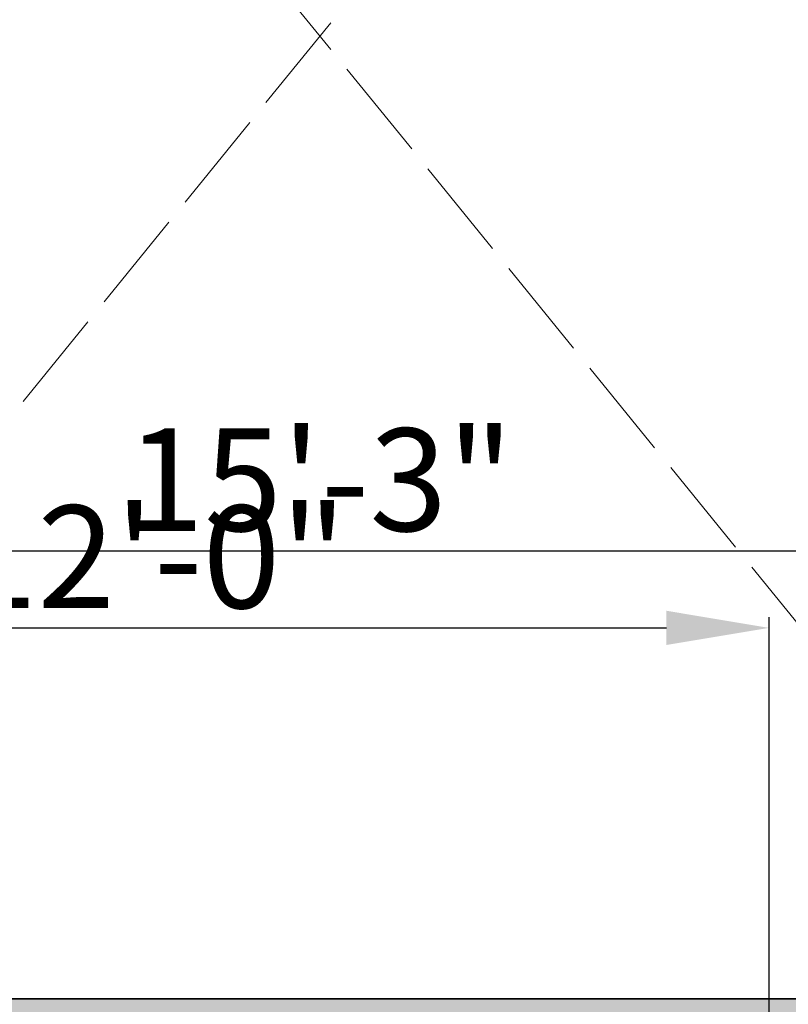
# Model space of a CAD drawing. Units: inches. Extents: x 2083 to 3317, y 1141 to 2115.
# Tile 82 of 256: x 2292 to 2382, y 1477 to 1592. Entities that reach past the tile are written whole.
import ezdxf

# ---------------------------------------------------------------- set-up
doc = ezdxf.new("R2010")
doc.units = ezdxf.units.IN
doc.linetypes.add('ACAD_ISO02W100', pattern=[15, 12, -3])
for name, color, linetype, lineweight in [('A-ANNO-DIMS', 2, 'Continuous', 18), ('A-FLOR-OPEN', 8, 'ACAD_ISO02W100', 13), ('A-WALL', 7, 'Continuous', 35)]:
    doc.layers.add(name, color=color, linetype=linetype, lineweight=lineweight)
doc.layers.add('A-WALL-PATT', color=251, linetype='Continuous', lineweight=13, true_color=0x636466)
doc.styles.get("Standard").update_dxf_attribs({"font": 'arial.ttf'})
doc.dimstyles.new('ISO-25', dxfattribs={"dimtxt": 12, "dimasz": 12, "dimexe": 1.25, "dimexo": 0.625, "dimtad": 1, "dimlunit": 3, "dimtxsty": 'Standard', "dimcen": 2.5, "dimadec": 0, "dimazin": 0, "dimtfac": 1, "dimtmove": 0, "dimatfit": 3, "dimfxl": 1, "dimarcsym": 0})

# ---------------------------------------------------------------- blocks, each defined once
blk = doc.blocks.new('*D30')
at = {"layer": 'A-ANNO-DIMS', "color": 0, "lineweight": -2, "transparency": 16777216}
for p, q in [((2240.02, 1445.27), (2240.02, 1448.05)), ((2254.33, 1445.27), (2254.33, 1448.05)), ((2228.02, 1446.8), (2216.02, 1446.8)), ((2240.02, 1446.8), (2254.33, 1446.8)), ((2266.33, 1446.8), (2413.76, 1446.8))]:
    blk.add_line(p, q, dxfattribs=at)
at = {"layer": 'A-ANNO-DIMS', "color": 0, "transparency": 16777216}
for points in [[(2228.02, 1448.8), (2228.02, 1444.8), (2240.02, 1446.8)], [(2266.33, 1448.8), (2266.33, 1444.8), (2254.33, 1446.8)]]:
    blk.add_solid(points, dxfattribs=at)
at = {"layer": 'Defpoints', "color": 0, "transparency": 16777216}
for p in [(2254.33, 1446.8), (2240.02, 1444.65), (2254.33, 1444.65)]:
    blk.add_point(p, dxfattribs=at)
at = {"layer": 'A-ANNO-DIMS', "color": 0, "transparency": 16777216, "insert": (2346.05, 1453.63), "char_height": 12, "attachment_point": 5}
blk.add_mtext('WC 1\'-2 1/2" TYP.', dxfattribs=at)
blk = doc.blocks.new('*D45')
at = {"layer": 'A-ANNO-DIMS', "color": 0, "lineweight": -2, "transparency": 16777216}
for p, q in [((2235.96, 1478.39), (2235.96, 1531.36)), ((2418.96, 1478.39), (2418.96, 1531.36)), ((2247.96, 1530.11), (2406.96, 1530.11))]:
    blk.add_line(p, q, dxfattribs=at)
at = {"layer": 'A-ANNO-DIMS', "color": 0, "transparency": 16777216}
for points in [[(2247.96, 1532.11), (2247.96, 1528.11), (2235.96, 1530.11)], [(2406.96, 1532.11), (2406.96, 1528.11), (2418.96, 1530.11)]]:
    blk.add_solid(points, dxfattribs=at)
at = {"layer": 'Defpoints', "color": 0, "transparency": 16777216}
for p in [(2418.96, 1530.11), (2235.96, 1477.76), (2418.96, 1477.76)]:
    blk.add_point(p, dxfattribs=at)
at = {"layer": 'A-ANNO-DIMS', "color": 0, "transparency": 16777216, "insert": (2327.46, 1536.87), "char_height": 12, "attachment_point": 5}
blk.add_mtext('15\'-3"', dxfattribs=at)
blk = doc.blocks.new('*D62')
at = {"layer": 'A-ANNO-DIMS', "color": 0, "lineweight": -2, "transparency": 16777216}
for p, q in [((2235.96, 1469.39), (2235.96, 1522.36)), ((2379.96, 1469.39), (2379.96, 1522.36)), ((2247.96, 1521.11), (2367.96, 1521.11))]:
    blk.add_line(p, q, dxfattribs=at)
at = {"layer": 'A-ANNO-DIMS', "color": 0, "transparency": 16777216}
for points in [[(2247.96, 1523.11), (2247.96, 1519.11), (2235.96, 1521.11)], [(2367.96, 1523.11), (2367.96, 1519.11), (2379.96, 1521.11)]]:
    blk.add_solid(points, dxfattribs=at)
at = {"layer": 'Defpoints', "color": 0, "transparency": 16777216}
for p in [(2379.96, 1521.11), (2235.96, 1468.76), (2379.96, 1468.76)]:
    blk.add_point(p, dxfattribs=at)
at = {"layer": 'A-ANNO-DIMS', "color": 0, "transparency": 16777216, "insert": (2307.96, 1527.86), "char_height": 12, "attachment_point": 5}
blk.add_mtext('12\'-0"', dxfattribs=at)

msp = doc.modelspace()

# ---------------------------------------------------------------- hatches: boundary and pattern name
at = {"layer": 'A-WALL-PATT'}
h = msp.add_hatch(color=256, dxfattribs=at)
h.dxf.hatch_style = 1
h.paths.add_polyline_path([(3126.96, 2020.761), (2748.96, 2020.761), (2604.96, 2020.761), (2226.96, 2020.761), (2226.96, 1702.761), (2466.96, 1702.761), (2466.96, 1582.761), (2418.96, 1582.761), (2418.96, 1477.761), (2226.96, 1477.761), (2226.96, 1263.261), (2544.96, 1263.261), (2544.96, 1411.761), (2604.96, 1411.761), (2685.96, 1411.761), (2685.96, 1420.761), (2604.96, 1420.761), (2604.96, 1573.761), (2604.96, 1702.761), (2604.96, 2011.761), (2748.96, 2011.761), (2748.96, 1702.761), (2862.96, 1702.761), (2862.96, 1621.761), (2871.96, 1621.761), (2871.96, 1702.761), (2883.96, 1702.761), (2883.96, 1706.939, -0.0264593), (2883.96, 1711.761), (2757.96, 1711.761), (2757.96, 1807.761), (2787.96, 1807.761), (2787.96, 1812.261), (2757.96, 1812.261), (2757.96, 2011.761), (2877.96, 2011.761), (2877.96, 1812.261), (2847.96, 1812.261), (2847.96, 1807.761), (2889.836, 1807.761), (2889.836, 1812.261), (2882.46, 1812.261), (2882.46, 2011.761), (3117.96, 2011.761), (3117.96, 1812.261), (2937.836, 1812.261), (2937.836, 1807.761), (2995.71, 1807.761), (2995.71, 1796.118), (3000.21, 1796.118), (3000.21, 1807.761), (3117.96, 1807.761), (3117.96, 1711.761), (3000.21, 1711.761), (3000.21, 1760.118), (2998.573, 1760.118, -0.020711), (2995.71, 1760.118), (2995.71, 1711.761), (2931.96, 1711.761), (2931.96, 1702.761), (3126.96, 1702.761)])
h.paths.add_polyline_path([(2471.46, 2011.761), (2471.46, 1810.011), (2462.717, 1810.011), (2462.717, 1805.511), (2505.96, 1805.511), (2505.96, 1810.011), (2475.96, 1810.011), (2475.96, 2011.761), (2595.96, 2011.761), (2595.96, 1810.011), (2565.96, 1810.011), (2565.96, 1805.511), (2595.96, 1805.511), (2595.96, 1711.761), (2235.96, 1711.761), (2235.96, 1805.511), (2353.71, 1805.511), (2353.71, 1796.054), (2358.21, 1796.054), (2358.21, 1805.511), (2414.717, 1805.511), (2414.717, 1810.011), (2235.96, 1810.011), (2235.96, 2011.761)], flags=16)
h.paths.add_polyline_path([(2270.205, 1994.61), (2270.205, 1970.61), (2246.205, 1970.61), (2246.205, 1994.61)], flags=0)
edge = h.paths.add_edge_path(flags=0)
edge.add_ellipse((2332.027, 1899.798), major_axis=(-3.043, 3.043), ratio=0.1682525, start_angle=-161.33217, end_angle=-156.30711, ccw=False)
edge.add_ellipse((2333.082, 1898.744), major_axis=(-1.055, 1.055), ratio=0.4535321, start_angle=-123.37102, end_angle=-94.15911)
edge = h.paths.add_edge_path(flags=0)
edge.add_ellipse((2332.027, 1968.876), major_axis=(3.043, 3.043), ratio=0.1682525, start_angle=18.66783, end_angle=23.69289)
edge.add_spline(control_points=[(2332.926, 1970.691), (2332.227, 1970.336), (2330.894, 1969.659), (2328.413, 1970.932), (2327.204, 1967.749), (2324.71, 1969.956), (2322.533, 1967.012), (2320.013, 1971.296), (2317.68, 1968.158), (2316.041, 1967.102), (2315.427, 1966.81)], knot_values=[0, 0, 0, 0, 2.2670587, 4.3245589, 6.6855835, 8.8786411, 11.121502, 14.300359, 17.7552837, 19.732645, 19.732645, 19.732645, 19.732645], degree=3, periodic=0)
edge.add_ellipse((2332.027, 1968.876), major_axis=(3.043, 3.043), ratio=0.1682525, start_angle=18.66783, end_angle=23.69289, ccw=False)
edge.add_ellipse((2333.082, 1969.931), major_axis=(1.055, 1.055), ratio=0.4535321, start_angle=56.62898, end_angle=85.84089, ccw=False)
edge = h.paths.add_edge_path(flags=0)
edge.add_spline(control_points=[(2296.428, 1967.988), (2293.628, 1965.336), (2287.704, 1959.727), (2299.744, 1949.996), (2294.533, 1935.669), (2290.573, 1920.604), (2293.394, 1909.974), (2296.185, 1904.967)], knot_values=[0.0991853, 0.0991853, 0.0991853, 0.0991853, 0.3453009, 0.6198217, 0.9826526, 1.3860932, 1.8105546, 1.8105546, 1.8105546, 1.8105546], degree=3, periodic=0)
edge.add_spline(control_points=[(2296.185, 1904.967), (2297.384, 1902.619), (2298.001, 1901.949), (2298.553, 1901.468)], knot_values=[0.0062457, 0.0062457, 0.0062457, 0.0062457, 0.0554759, 0.0554759, 0.0554759, 0.0554759], degree=3, periodic=0)
edge.add_spline(control_points=[(2298.553, 1901.468), (2297.259, 1900.923), (2295.225, 1900.232), (2293.06, 1900.614), (2292.101, 1900.788), (2292.09, 1900.791)], knot_values=[0.3128349, 0.3128349, 0.3128349, 0.3128349, 0.4017797, 0.4749867, 0.4759027, 0.4759027, 0.4759027, 0.4759027], degree=3, periodic=0)
edge.add_arc((2292.794, 1904.664), 3.937, 215.4209, 259.69818, ccw=False)
edge.add_spline(control_points=[(2289.585, 1902.382), (2289.477, 1902.535), (2289.368, 1902.688), (2289.261, 1902.841)], knot_values=[0.1028719, 0.1028719, 0.1028719, 0.1028719, 0.1168958, 0.1168958, 0.1168958, 0.1168958], degree=3, periodic=0)
edge.add_spline(control_points=[(2289.261, 1902.841), (2288.687, 1902.55), (2287.64, 1902.02), (2285.881, 1901.874), (2283.853, 1901.504), (2281.72, 1899.711), (2278.467, 1899.493), (2276.157, 1901.883), (2272.259, 1899.804), (2267.778, 1901.843), (2262.244, 1900.184), (2257.415, 1901.782), (2254.318, 1900.726), (2253.178, 1900.337)], knot_values=[0, 0, 0, 0, 1.9079767, 3.4771759, 5.261074, 7.9728515, 11.6802485, 13.7179214, 16.9395917, 22.789562, 27.5025027, 33.5952153, 37.1456181, 37.1456181, 37.1456181, 37.1456181], degree=3, periodic=0)
edge.add_line((2253.178, 1900.337), (2250.244, 1902.841))
edge.add_line((2250.244, 1902.841), (2250.244, 1965.833))
edge.add_line((2250.244, 1965.833), (2253.178, 1968.337))
edge.add_spline(control_points=[(2253.178, 1968.337), (2254.318, 1967.948), (2257.415, 1966.892), (2262.244, 1968.49), (2267.778, 1966.831), (2271.527, 1968.537), (2273.876, 1967.828), (2274.207, 1967.728)], knot_values=[0, 0, 0, 0, 0.0901802, 0.2449351, 0.3646438, 0.5132331, 0.5378548, 0.5378548, 0.5378548, 0.5378548], degree=3, periodic=0)
edge.add_arc((2274.353, 1963.793), 3.937, 72.05113, 92.12795, ccw=False)
edge.add_arc((2281.297, 1985.23), 18.596, 252.05113, 288.56572)
edge.add_arc((2292.317, 1956.029), 12.646, 71.02679, 113.77822, ccw=False)
edge = h.paths.add_edge_path(flags=0)
edge.add_spline(control_points=[(2274.899, 1951.856), (2275.066, 1951.617), (2275.233, 1951.377), (2275.398, 1951.136)], knot_values=[1.4099157, 1.4099157, 1.4099157, 1.4099157, 1.4315903, 1.4315903, 1.4315903, 1.4315903], degree=3, periodic=0)
edge.add_spline(control_points=[(2275.398, 1951.136), (2275.792, 1950.562), (2276.179, 1949.984), (2276.546, 1949.397)], knot_values=[1.3582378, 1.3582378, 1.3582378, 1.3582378, 1.4099157, 1.4099157, 1.4099157, 1.4099157], degree=3, periodic=0)
edge.add_line((2276.546, 1949.397), (2277.437, 1947.862))
edge.add_spline(control_points=[(2277.437, 1947.862), (2276.304, 1945.673), (2274.64, 1942.427), (2274.632, 1938.094), (2272.799, 1930.852), (2274.356, 1943.897), (2275.948, 1947.923), (2276.546, 1949.397)], knot_values=[0.0056315, 0.0056315, 0.0056315, 0.0056315, 0.1860139, 0.2660015, 0.3570872, 0.5963902, 0.7397317, 0.7397317, 0.7397317, 0.7397317], degree=3, periodic=0)
edge.add_spline(control_points=[(2276.546, 1949.397), (2276.179, 1949.984), (2275.792, 1950.562), (2275.398, 1951.136)], knot_values=[1.3582378, 1.3582378, 1.3582378, 1.3582378, 1.4099157, 1.4099157, 1.4099157, 1.4099157], degree=3, periodic=0)
edge.add_spline(control_points=[(2275.398, 1951.136), (2274.943, 1950.08), (2274.208, 1948.025), (2273.935, 1944.851), (2272.469, 1937.627), (2273.466, 1945.696), (2274.701, 1951.059), (2274.899, 1951.856)], knot_values=[0.1043639, 0.1043639, 0.1043639, 0.1043639, 0.1896363, 0.2696239, 0.3607096, 0.6000126, 0.6446217, 0.6446217, 0.6446217, 0.6446217], degree=3, periodic=0)
h.paths.add_polyline_path([(2269.168, 1963.128, -0.3575267), (2268.171, 1960.976, -0.0925607), (2268.171, 1939.436, -0.3575267), (2269.168, 1937.285, -0.3575267), (2267.016, 1938.282, -0.1647847), (2254.686, 1938.282, -0.3575267), (2252.534, 1937.285, -0.3575267), (2253.531, 1939.436, -0.0925607), (2253.531, 1960.976, -0.3575267), (2252.534, 1963.128, -0.3575267), (2254.686, 1962.131, -0.1647847), (2267.016, 1962.131, -0.3575267)], flags=0)
h.paths.add_polyline_path([(2248.874, 1967.802), (2248.874, 1957.028), (2249.458, 1957.028), (2249.458, 1911.647), (2248.874, 1911.647), (2248.874, 1900.873), (2246.512, 1900.873, 0.1973271), (2244.15, 1902.457), (2244.15, 1966.218, 0.1973271), (2246.512, 1967.802)], flags=0)
h.paths.add_polyline_path([(2269.168, 1931.389, -0.3575267), (2268.171, 1929.238, -0.0925607), (2268.171, 1907.698, -0.3575267), (2269.168, 1905.547, -0.3575267), (2267.016, 1906.544, -0.1647847), (2254.686, 1906.544, -0.3575267), (2252.534, 1905.547, -0.3575267), (2253.531, 1907.698, -0.0925607), (2253.531, 1929.238, -0.3575267), (2252.534, 1931.389, -0.3575267), (2254.686, 1930.392, -0.1647847), (2267.016, 1930.392, -0.3575267)], flags=0)
edge = h.paths.add_edge_path(flags=0)
edge.add_spline(control_points=[(2276.197, 1906.724), (2276.168, 1909.029), (2276.114, 1913.372), (2270.598, 1924.925), (2273.905, 1919.013), (2275.922, 1916.262), (2275.475, 1912.402), (2277.258, 1910.381), (2276.696, 1908.225), (2276.646, 1906.813), (2276.618, 1906.008)], knot_values=[0, 0, 0, 0, 8.6102597, 16.2212739, 18.8430575, 23.8048978, 27.4408283, 29.3561016, 31.2034776, 33.6506866, 33.6506866, 33.6506866, 33.6506866], degree=3, periodic=0)
edge.add_spline(control_points=[(2276.618, 1906.008), (2276.623, 1905.624), (2276.498, 1904.629), (2275.442, 1903.855), (2274.937, 1903.08), (2274.859, 1902.841)], knot_values=[0.1564884, 0.1564884, 0.1564884, 0.1564884, 0.1843975, 0.2313765, 0.2505985, 0.2505985, 0.2505985, 0.2505985], degree=3, periodic=0)
edge.add_line((2274.859, 1902.841), (2276.506, 1902.841))
edge.add_spline(control_points=[(2276.506, 1902.841), (2276.788, 1903.085), (2277.665, 1904.125), (2278.25, 1904.341), (2277.654, 1908.527), (2278.156, 1906.228), (2278.1, 1905.286), (2278.847, 1904.069), (2277.857, 1903.415), (2277.874, 1902.991), (2277.904, 1902.841)], knot_values=[0.0595743, 0.0595743, 0.0595743, 0.0595743, 0.0807529, 0.1037415, 0.1697201, 0.1760361, 0.2071372, 0.2404744, 0.2623409, 0.2736605, 0.2736605, 0.2736605, 0.2736605], degree=3, periodic=0)
edge.add_line((2277.904, 1902.841), (2280.03, 1902.841))
edge.add_spline(control_points=[(2280.03, 1902.841), (2279.888, 1903.088), (2279.499, 1903.982), (2280.152, 1905.939), (2278.104, 1909.658), (2279.762, 1907.185), (2280.328, 1904.875), (2280.485, 1903.49), (2281.463, 1903.249), (2281.758, 1902.936), (2281.834, 1902.841)], knot_values=[0.013856, 0.013856, 0.013856, 0.013856, 0.0348738, 0.0888667, 0.1078792, 0.1267378, 0.158714, 0.1937575, 0.2174868, 0.2267221, 0.2267221, 0.2267221, 0.2267221], degree=3, periodic=0)
edge.add_spline(control_points=[(2281.834, 1902.841), (2281.788, 1902.827), (2281.647, 1902.783), (2281.396, 1902.859), (2281.088, 1902.985), (2280.721, 1903.061), (2280.333, 1903.026), (2280.125, 1902.899), (2280.03, 1902.841)], knot_values=[0, 0, 0, 0, 0.1441304, 0.435517, 0.7492759, 1.1530457, 1.5483707, 1.878348, 1.878348, 1.878348, 1.878348], degree=3, periodic=0)
edge.add_line((2280.03, 1902.841), (2277.904, 1902.841))
edge.add_spline(control_points=[(2277.904, 1902.841), (2277.893, 1902.796), (2277.865, 1902.68), (2277.607, 1902.687), (2277.274, 1902.801), (2276.838, 1902.62), (2276.584, 1902.789), (2276.506, 1902.841)], knot_values=[0, 0, 0, 0, 0.1271885, 0.3261988, 0.6280094, 1.2435704, 1.5153306, 1.5153306, 1.5153306, 1.5153306], degree=3, periodic=0)
edge.add_line((2276.506, 1902.841), (2274.859, 1902.841))
edge.add_spline(control_points=[(2274.859, 1902.841), (2274.814, 1902.899), (2274.725, 1903.013), (2274.493, 1903.119), (2274.244, 1902.961), (2273.937, 1903.185), (2273.614, 1902.983), (2273.408, 1902.883), (2273.322, 1902.841)], knot_values=[0, 0, 0, 0, 0.2184302, 0.4369566, 0.6879766, 0.9903786, 1.3983955, 1.6918498, 1.6918498, 1.6918498, 1.6918498], degree=3, periodic=0)
edge.add_spline(control_points=[(2273.322, 1902.841), (2273.617, 1903.446), (2274.274, 1904.538), (2276.027, 1904.574), (2276.207, 1906.584), (2276.197, 1906.724)], knot_values=[0.0122268, 0.0122268, 0.0122268, 0.0122268, 0.0594721, 0.1062177, 0.134458, 0.134458, 0.134458, 0.134458], degree=3, periodic=0)
h.paths.add_polyline_path([(2270.776, 1897.79), (2270.776, 1873.79), (2246.776, 1873.79), (2246.776, 1897.79)], flags=0)
h.paths.add_polyline_path([(2353.71, 1760.005), (2353.71, 1760.054), (2358.21, 1760.054, -0.033729)], flags=0)
h.paths.add_polyline_path([(2321.819, 1737.529), (2341.995, 1737.529, -0.4142136), (2343.203, 1736.321), (2343.203, 1721.021, -0.4142136), (2341.995, 1719.813), (2321.819, 1719.813, -0.4142136), (2320.611, 1721.021), (2320.611, 1736.321, -0.4142136)], flags=0)
h.paths.add_polyline_path([(2324.235, 1736.321), (2339.579, 1736.321, -0.4142136), (2341.995, 1733.905), (2341.995, 1725.45, -0.4142136), (2339.579, 1723.034), (2333.681, 1723.034), (2333.845, 1722.045, -0.8706461), (2335.425, 1721.826, -0.767327), (2333.923, 1721.423), (2331.291, 1721.423, -0.767327), (2329.788, 1721.826, -0.8706461), (2331.368, 1722.045), (2331.533, 1723.034), (2324.235, 1723.034, -0.4142136), (2321.819, 1725.45), (2321.819, 1733.905, -0.4142136)], flags=0)
h.paths.add_polyline_path([(2570.484, 1928.615), (2589.684, 1928.615), (2590.169, 1928.615), (2590.169, 1904.993), (2570.484, 1904.993)], flags=0)
h.paths.add_polyline_path([(2574.447, 1927.264, -1), (2572.829, 1927.264, -1)], flags=0)
h.paths.add_polyline_path([(2573.09, 1926.941), (2573.925, 1927.776), (2574.148, 1927.553), (2573.313, 1926.718)], flags=0)
h.paths.add_polyline_path([(2578.779, 1919.73, -1), (2571.592, 1919.73, -1)], flags=0)
h.paths.add_polyline_path([(2578.385, 1919.73, -1), (2571.985, 1919.73, -1)], flags=0)
h.paths.add_polyline_path([(2331.596, 1729.476, -1), (2333.618, 1729.476, -1)], flags=0)
h.paths.add_polyline_path([(2578.034, 1927.264, -1), (2576.416, 1927.264, -1)], flags=0)
h.paths.add_polyline_path([(2576.689, 1927.531), (2576.912, 1927.754), (2577.747, 1926.919), (2577.524, 1926.696)], flags=0)
h.paths.add_polyline_path([(2578.139, 1909.86, -1), (2572.232, 1909.86, -1)], flags=0)
h.paths.add_polyline_path([(2577.745, 1909.86, -1), (2572.625, 1909.86, -1)], flags=0)
h.paths.add_polyline_path([(2583.798, 1927.264, -1), (2582.179, 1927.264, -1)], flags=0)
h.paths.add_polyline_path([(2582.719, 1927.754), (2583.554, 1926.919), (2583.331, 1926.696), (2582.496, 1927.531)], flags=0)
h.paths.add_polyline_path([(2582.496, 1927.531), (2582.719, 1927.754), (2583.554, 1926.919), (2583.331, 1926.696)], flags=0)
h.paths.add_polyline_path([(2587.739, 1920.53, -1), (2581.832, 1920.53, -1)], flags=0)
h.paths.add_polyline_path([(2587.345, 1920.53, -1), (2582.225, 1920.53, -1)], flags=0)
h.paths.add_polyline_path([(2587.385, 1927.264, -1), (2585.766, 1927.264, -1)], flags=0)
h.paths.add_polyline_path([(2586.082, 1926.98), (2586.917, 1927.815), (2587.14, 1927.593), (2586.305, 1926.758)], flags=0)
h.paths.add_polyline_path([(2588.379, 1910.66, -1), (2581.192, 1910.66, -1)], flags=0)
h.paths.add_polyline_path([(2587.985, 1910.66, -1), (2581.585, 1910.66, -1)], flags=0)
h.paths.add_polyline_path([(2417.168, 1729.478), (2437.344, 1729.478, -0.4142136), (2438.552, 1728.27), (2438.552, 1712.969, -0.4142136), (2437.344, 1711.761), (2417.168, 1711.761, -0.4142136), (2415.96, 1712.969), (2415.96, 1728.27, -0.4142136)], flags=0)
h.paths.add_polyline_path([(2419.584, 1728.27), (2434.928, 1728.27, -0.4142136), (2437.344, 1725.854), (2437.344, 1717.398, -0.4142136), (2434.928, 1714.983), (2429.029, 1714.983), (2429.194, 1713.994, -0.8706461), (2430.774, 1713.775, -0.767327), (2429.271, 1713.372), (2426.64, 1713.372, -0.767327), (2425.137, 1713.775, -0.8706461), (2426.717, 1713.994), (2426.882, 1714.983), (2419.584, 1714.983, -0.4142136), (2417.168, 1717.398), (2417.168, 1725.854, -0.4142136)], flags=0)
h.paths.add_polyline_path([(2419.584, 1728.27), (2434.928, 1728.27, -0.4142136), (2437.344, 1725.854), (2437.344, 1717.398, -0.4142136), (2434.928, 1714.983), (2429.029, 1714.983), (2428.358, 1719.009), (2427.553, 1719.009), (2426.882, 1714.983), (2419.584, 1714.983, -0.4142136), (2417.168, 1717.398), (2417.168, 1725.854, -0.4142136)], flags=0)
h.paths.add_polyline_path([(2426.944, 1721.425, -1), (2428.967, 1721.425, -1)], flags=0)
h.paths.add_polyline_path([(2475.96, 1702.761), (2595.96, 1702.761), (2595.96, 1582.761), (2475.96, 1582.761)], flags=16)
h.paths.add_polyline_path([(2427.96, 1573.761), (2595.96, 1573.761), (2595.96, 1468.761), (2595.96, 1420.761), (2384.46, 1420.761), (2384.46, 1468.761), (2427.96, 1468.761)], flags=16)
h.paths.add_polyline_path([(2379.96, 1468.761), (2379.96, 1420.761), (2235.96, 1420.761), (2235.96, 1468.761)], flags=16)
h.paths.add_polyline_path([(2317.816, 1466.696), (2337.992, 1466.696, -0.4142136), (2339.2, 1465.488), (2339.2, 1450.187, -0.4142136), (2337.992, 1448.979), (2317.816, 1448.979, -0.4142136), (2316.608, 1450.187), (2316.608, 1465.488, -0.4142136)], flags=0)
h.paths.add_polyline_path([(2320.232, 1465.488), (2335.576, 1465.488, -0.4142136), (2337.992, 1463.072), (2337.992, 1454.616, -0.4142136), (2335.576, 1452.2), (2329.677, 1452.2), (2329.842, 1451.212, -0.8706461), (2331.422, 1450.992, -0.767327), (2329.92, 1450.59), (2327.288, 1450.59, -0.767327), (2325.785, 1450.992, -0.8706461), (2327.365, 1451.212), (2327.53, 1452.2), (2320.232, 1452.2, -0.4142136), (2317.816, 1454.616), (2317.816, 1463.072, -0.4142136)], flags=0)
h.paths.add_polyline_path([(2320.232, 1465.488), (2335.576, 1465.488, -0.4142136), (2337.992, 1463.072), (2337.992, 1454.616, -0.4142136), (2335.576, 1452.2), (2329.677, 1452.2), (2329.006, 1456.227), (2328.201, 1456.227), (2327.53, 1452.2), (2320.232, 1452.2, -0.4142136), (2317.816, 1454.616), (2317.816, 1463.072, -0.4142136)], flags=0)
h.paths.add_polyline_path([(2327.593, 1458.643, -1), (2329.615, 1458.643, -1)], flags=0)
h.paths.add_polyline_path([(2244.412, 1433.34), (2241.921, 1433.34, -0.4142136), (2240.018, 1435.244), (2240.018, 1440.953, -0.4142105), (2241.921, 1442.856), (2244.412, 1442.856, -1.9764724)], flags=0)
h.paths.add_polyline_path([(2245.357, 1434.398, -0.4142136), (2245.357, 1441.799, -2.1440985)], flags=0)
h.paths.add_polyline_path([(2535.96, 1416.261), (2535.96, 1272.261), (2235.96, 1272.261), (2235.96, 1416.261)], flags=16)
h.paths.add_polyline_path([(2260.12, 1384.293), (2260.12, 1362.039), (2237.865, 1362.039), (2237.865, 1384.293)], flags=0)
edge = h.paths.add_edge_path(flags=0)
edge.add_line((2318.252, 1362.093), (2318.146, 1362.001))
edge.add_ellipse((2317.445, 1360.431), major_axis=(2.822, 2.822), ratio=0.1682525, start_angle=18.66783, end_angle=20.94813, ccw=False)
edge.add_ellipse((2318.423, 1361.409), major_axis=(0.978, 0.978), ratio=0.4535321, start_angle=56.62898, end_angle=70.2262, ccw=False)
edge = h.paths.add_edge_path(flags=0)
edge.add_line((2319.107, 1295.571), (2319.015, 1295.677))
edge.add_ellipse((2317.445, 1296.378), major_axis=(-2.822, 2.822), ratio=0.1682525, start_angle=-161.33217, end_angle=-159.05187, ccw=False)
edge.add_ellipse((2318.423, 1295.4), major_axis=(-0.978, 0.978), ratio=0.4535321, start_angle=-123.37102, end_angle=-109.7738)
edge = h.paths.add_edge_path(flags=0)
edge.add_spline(control_points=[(2284.21, 1301.17), (2284.581, 1300.445), (2284.891, 1299.892), (2285.16, 1299.461)], knot_values=[0.0390658, 0.0390658, 0.0390658, 0.0390658, 0.0554759, 0.0554759, 0.0554759, 0.0554759], degree=3, periodic=0)
edge.add_line((2285.16, 1299.461), (2284.21, 1301.17))
edge = h.paths.add_edge_path(flags=0)
edge.add_line((2280.412, 1297.298), (2283.37, 1297.036))
edge.add_line((2283.37, 1297.036), (2286.406, 1297.926))
edge.add_spline(control_points=[(2286.406, 1297.926), (2285.305, 1297.463), (2284.345, 1297.129), (2283.37, 1297.036)], knot_values=[0.3943688, 0.3943688, 0.3943688, 0.3943688, 0.4759027, 0.4759027, 0.4759027, 0.4759027], degree=3, periodic=0)
edge.add_spline(control_points=[(2283.37, 1297.036), (2283.281, 1297.028), (2282.316, 1296.957), (2281.313, 1297.134), (2280.423, 1297.296), (2280.412, 1297.298)], knot_values=[0.3128349, 0.3128349, 0.3128349, 0.3128349, 0.3202458, 0.3934528, 0.3943688, 0.3943688, 0.3943688, 0.3943688], degree=3, periodic=0)
edge = h.paths.add_edge_path(flags=0)
edge.add_line((2284.436, 1359.607), (2280.446, 1355.328))
edge.add_line((2280.446, 1355.328), (2279.58, 1351.018))
edge.add_line((2279.58, 1351.018), (2282.413, 1346.58))
edge.add_spline(control_points=[(2282.413, 1346.58), (2283.153, 1345.589), (2284.253, 1344.029), (2284.801, 1342.387), (2284.935, 1341.806)], knot_values=[1.2400982, 1.2400982, 1.2400982, 1.2400982, 1.3328922, 1.3827123, 1.3827123, 1.3827123, 1.3827123], degree=3, periodic=0)
edge.add_spline(control_points=[(2284.935, 1341.806), (2285.319, 1340.141), (2285.233, 1338.409), (2284.91, 1336.654)], knot_values=[1.0974841, 1.0974841, 1.0974841, 1.0974841, 1.2400982, 1.2400982, 1.2400982, 1.2400982], degree=3, periodic=0)
edge.add_spline(control_points=[(2284.91, 1336.654), (2284.587, 1334.899), (2284.027, 1333.12), (2283.463, 1331.361)], knot_values=[0.9548699, 0.9548699, 0.9548699, 0.9548699, 1.0974841, 1.0974841, 1.0974841, 1.0974841], degree=3, periodic=0)
edge.add_line((2283.463, 1331.361), (2281.89, 1326.153))
edge.add_line((2281.89, 1326.153), (2280.756, 1321.056))
edge.add_line((2280.756, 1321.056), (2280.299, 1316.002))
edge.add_line((2280.299, 1316.002), (2280.716, 1310.95))
edge.add_line((2280.716, 1310.95), (2282.028, 1305.972))
edge.add_line((2282.028, 1305.972), (2284.21, 1301.17))
edge.add_spline(control_points=[(2284.21, 1301.17), (2283.341, 1302.73), (2282.612, 1304.336), (2282.028, 1305.972)], knot_values=[0.0991853, 0.0991853, 0.0991853, 0.0991853, 0.2417994, 0.2417994, 0.2417994, 0.2417994], degree=3, periodic=0)
edge.add_spline(control_points=[(2282.028, 1305.972), (2281.444, 1307.608), (2281.005, 1309.273), (2280.716, 1310.95)], knot_values=[0.2417994, 0.2417994, 0.2417994, 0.2417994, 0.3844135, 0.3844135, 0.3844135, 0.3844135], degree=3, periodic=0)
edge.add_spline(control_points=[(2280.716, 1310.95), (2280.433, 1312.588), (2280.289, 1314.277), (2280.299, 1315.962), (2280.299, 1316.002)], knot_values=[0.3844135, 0.3844135, 0.3844135, 0.3844135, 0.5236467, 0.5270276, 0.5270276, 0.5270276, 0.5270276], degree=3, periodic=0)
edge.add_spline(control_points=[(2280.299, 1316.002), (2280.312, 1317.687), (2280.478, 1319.368), (2280.756, 1321.056)], knot_values=[0.5270276, 0.5270276, 0.5270276, 0.5270276, 0.6696417, 0.6696417, 0.6696417, 0.6696417], degree=3, periodic=0)
edge.add_spline(control_points=[(2280.756, 1321.056), (2281.035, 1322.744), (2281.426, 1324.44), (2281.89, 1326.153)], knot_values=[0.6696417, 0.6696417, 0.6696417, 0.6696417, 0.8122558, 0.8122558, 0.8122558, 0.8122558], degree=3, periodic=0)
edge.add_spline(control_points=[(2281.89, 1326.153), (2282.264, 1327.533), (2282.788, 1329.262), (2283.353, 1331.018), (2283.463, 1331.361)], knot_values=[0.8122558, 0.8122558, 0.8122558, 0.8122558, 0.9270873, 0.9548699, 0.9548699, 0.9548699, 0.9548699], degree=3, periodic=0)
edge.add_line((2283.463, 1331.361), (2284.91, 1336.654))
edge.add_line((2284.91, 1336.654), (2284.935, 1341.806))
edge.add_line((2284.935, 1341.806), (2282.413, 1346.58))
edge.add_spline(control_points=[(2282.413, 1346.58), (2281.275, 1348.104), (2280.078, 1349.57), (2279.58, 1351.018)], knot_values=[1.3827123, 1.3827123, 1.3827123, 1.3827123, 1.5253264, 1.5253264, 1.5253264, 1.5253264], degree=3, periodic=0)
edge.add_spline(control_points=[(2279.58, 1351.018), (2279.443, 1351.415), (2279.136, 1352.857), (2279.735, 1354.29), (2280.446, 1355.328)], knot_values=[1.5253264, 1.5253264, 1.5253264, 1.5253264, 1.564439, 1.6679405, 1.6679405, 1.6679405, 1.6679405], degree=3, periodic=0)
edge.add_spline(control_points=[(2280.446, 1355.328), (2281.426, 1356.758), (2282.931, 1358.183), (2284.436, 1359.607)], knot_values=[1.6679405, 1.6679405, 1.6679405, 1.6679405, 1.8105546, 1.8105546, 1.8105546, 1.8105546], degree=3, periodic=0)
edge.add_arc((2280.623, 1348.518), 11.726, 71.02679, 113.77822)
edge.add_arc((2270.405, 1375.595), 17.244, 252.05113, 288.56572, ccw=False)
edge.add_arc((2263.966, 1355.718), 3.651, 72.05113, 92.12795)
edge.add_arc((2263.966, 1355.718), 3.651, 92.12795, 177.98513)
edge.add_spline(control_points=[(2260.318, 1355.846), (2260.26, 1354.221), (2260.551, 1350.187), (2262.999, 1346.766), (2264.473, 1344.649)], knot_values=[1.4315903, 1.4315903, 1.4315903, 1.4315903, 1.5641438, 1.7706953, 1.7706953, 1.7706953, 1.7706953], degree=3, periodic=0)
edge.add_line((2264.473, 1344.649), (2264.936, 1343.983))
edge.add_spline(control_points=[(2263.801, 1340.248), (2263.843, 1340.514), (2264.067, 1341.756), (2264.513, 1343.002), (2264.935, 1343.981)], knot_values=[0.5365702, 0.5365702, 0.5365702, 0.5365702, 0.5593494, 0.6446217, 0.6446217, 0.6446217, 0.6446217], degree=3, periodic=0)
edge.add_spline(control_points=[(2264.935, 1343.981), (2265.118, 1343.715), (2265.299, 1343.448), (2265.477, 1343.179)], knot_values=[1.3840767, 1.3840767, 1.3840767, 1.3840767, 1.4099157, 1.4099157, 1.4099157, 1.4099157], degree=3, periodic=0)
edge.add_spline(control_points=[(2265.477, 1343.179), (2265.655, 1342.911), (2265.829, 1342.641), (2265.999, 1342.369)], knot_values=[1.3582378, 1.3582378, 1.3582378, 1.3582378, 1.3840767, 1.3840767, 1.3840767, 1.3840767], degree=3, periodic=0)
edge.add_line((2265.999, 1342.369), (2266.826, 1340.946))
edge.add_spline(control_points=[(2266.826, 1340.946), (2268.894, 1337.09), (2271.398, 1325.843), (2270.516, 1310.569), (2275.919, 1301.861), (2277.79, 1299.199)], knot_values=[0.1168958, 0.1168958, 0.1168958, 0.1168958, 0.4729873, 1.0509689, 1.3137934, 1.3137934, 1.3137934, 1.3137934], degree=3, periodic=0)
edge.add_spline(control_points=[(2277.79, 1299.199), (2277.839, 1299.128), (2277.889, 1299.057), (2277.94, 1298.987)], knot_values=[0.1098839, 0.1098839, 0.1098839, 0.1098839, 0.1168958, 0.1168958, 0.1168958, 0.1168958], degree=3, periodic=0)
edge.add_line((2277.94, 1298.987), (2277.789, 1299.199))
edge.add_spline(control_points=[(2277.789, 1299.199), (2277.257, 1298.929), (2276.286, 1298.438), (2275.039, 1298.334), (2274.383, 1298.239), (2274.215, 1298.209)], knot_values=[33.1218702, 33.1218702, 33.1218702, 33.1218702, 35.0290557, 36.5982549, 37.1448269, 37.1448269, 37.1448269, 37.1448269], degree=3, periodic=0)
edge.add_line((2274.215, 1298.209), (2273.073, 1297.893))
edge.add_spline(control_points=[(2273.073, 1297.893), (2272.323, 1297.58), (2271.039, 1296.511), (2269.248, 1296.226), (2268.423, 1296.375)], knot_values=[26.5325843, 26.5325843, 26.5325843, 26.5325843, 29.198919, 31.8391012, 31.8391012, 31.8391012, 31.8391012], degree=3, periodic=0)
edge.add_line((2268.423, 1296.375), (2263.879, 1297.458))
edge.add_spline(control_points=[(2263.879, 1297.458), (2263.556, 1297.359), (2261.86, 1296.839), (2260.239, 1297.282), (2258.933, 1297.516)], knot_values=[15.9195506, 15.9195506, 15.9195506, 15.9195506, 16.9395917, 21.2260675, 21.2260675, 21.2260675, 21.2260675], degree=3, periodic=0)
edge.add_line((2258.933, 1297.516), (2254.055, 1297.329))
edge.add_spline(control_points=[(2254.055, 1297.329), (2253.756, 1297.296), (2252.114, 1297.165), (2250.462, 1297.544), (2249.13, 1297.668)], knot_values=[5.3065169, 5.3065169, 5.3065169, 5.3065169, 6.2764352, 10.6130337, 10.6130337, 10.6130337, 10.6130337], degree=3, periodic=0)
edge.add_line((2249.13, 1297.668), (2244.332, 1296.878))
edge.add_line((2244.332, 1296.878), (2241.611, 1299.199))
edge.add_line((2241.611, 1299.199), (2241.611, 1357.609))
edge.add_line((2241.611, 1357.609), (2244.332, 1359.931))
edge.add_line((2244.332, 1359.931), (2252.729, 1359.543))
edge.add_spline(control_points=[(2252.729, 1359.543), (2252.871, 1359.546), (2253.306, 1359.548), (2253.74, 1359.514), (2254.032, 1359.482)], knot_values=[0.233291, 0.233291, 0.233291, 0.233291, 0.2449351, 0.2689274, 0.2689274, 0.2689274, 0.2689274], degree=3, periodic=0)
edge.add_line((2254.032, 1359.482), (2259.587, 1359.416))
edge.add_spline(control_points=[(2259.587, 1359.416), (2260.677, 1359.629), (2262.073, 1359.897), (2263.524, 1359.459), (2263.83, 1359.366)], knot_values=[0.4225164, 0.4225164, 0.4225164, 0.4225164, 0.5132331, 0.5378548, 0.5378548, 0.5378548, 0.5378548], degree=3, periodic=0)
edge.add_arc((2263.966, 1355.718), 3.651, 72.05113, 92.12795, ccw=False)
edge.add_arc((2270.405, 1375.595), 17.244, 252.05113, 288.56572)
edge.add_arc((2280.623, 1348.518), 11.726, 71.02679, 113.77822, ccw=False)
h.paths.add_polyline_path([(2240.341, 1359.435), (2240.341, 1349.444), (2240.882, 1349.444), (2240.882, 1307.365), (2240.341, 1307.365), (2240.341, 1297.374), (2238.15, 1297.374, 0.1973271), (2235.96, 1298.843), (2235.96, 1357.966, 0.1973271), (2238.15, 1359.435)], flags=0)
h.paths.add_polyline_path([(2259.158, 1355.101, -0.3575267), (2258.233, 1353.106, -0.0925607), (2258.233, 1333.133, -0.3575267), (2259.158, 1331.138, -0.3575267), (2257.163, 1332.062, -0.1647847), (2245.729, 1332.062, -0.3575267), (2243.735, 1331.138, -0.3575267), (2244.659, 1333.133, -0.0925607), (2244.659, 1353.106, -0.3575267), (2243.735, 1355.101, -0.3575267), (2245.729, 1354.176, -0.1647847), (2257.163, 1354.176, -0.3575267)], flags=0)
edge = h.paths.add_edge_path(flags=0)
edge.add_line((2265.999, 1342.369), (2266.826, 1340.946))
edge.add_line((2266.826, 1340.946), (2265.308, 1337.814))
edge.add_line((2265.308, 1337.814), (2264.358, 1334.653))
edge.add_line((2264.358, 1334.653), (2264.262, 1333.8))
edge.add_spline(control_points=[(2264.262, 1333.8), (2264.208, 1333.187), (2264.162, 1332.366), (2264.007, 1331.414), (2263.969, 1331.202)], knot_values=[0.4644442, 0.4644442, 0.4644442, 0.4644442, 0.5166905, 0.5316081, 0.5316081, 0.5316081, 0.5316081], degree=3, periodic=0)
edge.add_spline(control_points=[(2263.969, 1331.202), (2263.775, 1330.119), (2263.424, 1328.791), (2263.257, 1328.531), (2263.234, 1328.515)], knot_values=[0.3726816, 0.3726816, 0.3726816, 0.3726816, 0.4488497, 0.4644442, 0.4644442, 0.4644442, 0.4644442], degree=3, periodic=0)
edge.add_spline(control_points=[(2263.234, 1328.515), (2263.096, 1328.42), (2263.131, 1329.301), (2263.275, 1330.616)], knot_values=[0.2809191, 0.2809191, 0.2809191, 0.2809191, 0.3726816, 0.3726816, 0.3726816, 0.3726816], degree=3, periodic=0)
edge.add_spline(control_points=[(2263.275, 1330.616), (2263.419, 1331.93), (2263.672, 1333.677), (2263.97, 1335.315)], knot_values=[0.1891566, 0.1891566, 0.1891566, 0.1891566, 0.2809191, 0.2809191, 0.2809191, 0.2809191], degree=3, periodic=0)
edge.add_spline(control_points=[(2263.97, 1335.315), (2264.1, 1336.032), (2264.419, 1337.622), (2264.755, 1338.864), (2264.947, 1339.491)], knot_values=[0.097394, 0.097394, 0.097394, 0.097394, 0.1375775, 0.1891566, 0.1891566, 0.1891566, 0.1891566], degree=3, periodic=0)
edge.add_spline(control_points=[(2264.947, 1339.491), (2265.29, 1340.606), (2265.644, 1341.494), (2265.999, 1342.369)], knot_values=[0.0056315, 0.0056315, 0.0056315, 0.0056315, 0.097394, 0.097394, 0.097394, 0.097394], degree=3, periodic=0)
h.paths.add_polyline_path([(2259.158, 1325.671, -0.3575267), (2258.233, 1323.676, -0.0925607), (2258.233, 1303.703, -0.3575267), (2259.158, 1301.708, -0.3575267), (2257.163, 1302.633, -0.1647847), (2245.729, 1302.633, -0.3575267), (2243.735, 1301.708, -0.3575267), (2244.659, 1303.703, -0.0925607), (2244.659, 1323.676, -0.3575267), (2243.735, 1325.671, -0.3575267), (2245.729, 1324.747, -0.1647847), (2257.163, 1324.747, -0.3575267)], flags=0)
edge = h.paths.add_edge_path(flags=0)
edge.add_spline(control_points=[(2261.709, 1317.311), (2261.679, 1317.418), (2261.762, 1317.389), (2262.491, 1316.09), (2262.962, 1315.301)], knot_values=[14.9558607, 14.9558607, 14.9558607, 14.9558607, 16.2212739, 18.6948259, 18.6948259, 18.6948259, 18.6948259], degree=3, periodic=0)
edge.add_spline(control_points=[(2262.962, 1315.301), (2262.99, 1315.254), (2263.702, 1314.067), (2264.349, 1313.127), (2264.73, 1312.164)], knot_values=[18.6948259, 18.6948259, 18.6948259, 18.6948259, 18.8430575, 22.433791, 22.433791, 22.433791, 22.433791], degree=3, periodic=0)
edge.add_spline(control_points=[(2264.73, 1312.164), (2264.876, 1311.796), (2265.177, 1310.77), (2265.143, 1309.559), (2265.248, 1308.824)], knot_values=[22.433791, 22.433791, 22.433791, 22.433791, 23.8048978, 26.1727562, 26.1727562, 26.1727562, 26.1727562], degree=3, periodic=0)
edge.add_line((2265.248, 1308.824), (2265.851, 1307.172))
edge.add_spline(control_points=[(2265.851, 1307.172), (2266.065, 1306.822), (2266.384, 1306.332), (2266.424, 1305.781), (2266.42, 1305.611)], knot_values=[28.0625624, 28.0625624, 28.0625624, 28.0625624, 29.3561016, 29.9117214, 29.9117214, 29.9117214, 29.9117214], degree=3, periodic=0)
edge.add_spline(control_points=[(2266.42, 1305.611), (2266.416, 1305.433), (2266.394, 1305.25), (2266.365, 1305.066)], knot_values=[29.9117214, 29.9117214, 29.9117214, 29.9117214, 30.4978371, 30.4978371, 30.4978371, 30.4978371], degree=3, periodic=0)
edge.add_line((2266.365, 1305.066), (2266.066, 1302.136))
edge.add_spline(control_points=[(2266.066, 1302.136), (2266.071, 1301.78), (2265.998, 1301.2), (2265.663, 1300.759), (2265.509, 1300.586)], knot_values=[0.1564884, 0.1564884, 0.1564884, 0.1564884, 0.1843975, 0.2035434, 0.2035434, 0.2035434, 0.2035434], degree=3, periodic=0)
edge.add_line((2265.509, 1300.586), (2264.435, 1299.199))
edge.add_line((2264.435, 1299.199), (2265.962, 1299.199))
edge.add_line((2265.962, 1299.199), (2267.336, 1301.175))
edge.add_line((2267.336, 1301.175), (2267.312, 1301.986))
edge.add_spline(control_points=[(2267.312, 1301.986), (2267.261, 1302.862), (2267.16, 1303.737), (2267.271, 1303.326)], knot_values=[0.1262286, 0.1262286, 0.1262286, 0.1262286, 0.1666174, 0.1666174, 0.1666174, 0.1666174], degree=3, periodic=0)
edge.add_spline(control_points=[(2267.271, 1303.326), (2267.28, 1303.294), (2267.31, 1303.175), (2267.373, 1302.884), (2267.406, 1302.683), (2267.418, 1302.601)], knot_values=[0.1666174, 0.1666174, 0.1666174, 0.1666174, 0.1697201, 0.1760361, 0.1807647, 0.1807647, 0.1807647, 0.1807647], degree=3, periodic=0)
edge.add_spline(control_points=[(2267.744, 1300.988), (2267.688, 1301.151), (2267.481, 1301.657), (2267.484, 1302.145), (2267.418, 1302.601)], knot_values=[0.1807647, 0.1807647, 0.1807647, 0.1807647, 0.1937665, 0.2201389, 0.2201389, 0.2201389, 0.2201389], degree=3, periodic=0)
edge.add_line((2267.418, 1302.601), (2267.744, 1300.988))
edge.add_spline(control_points=[(2267.744, 1300.988), (2267.832, 1300.732), (2267.932, 1300.31), (2267.555, 1299.975), (2267.429, 1299.829)], knot_values=[0.2201389, 0.2201389, 0.2201389, 0.2201389, 0.2404744, 0.2548903, 0.2548903, 0.2548903, 0.2548903], degree=3, periodic=0)
edge.add_line((2267.429, 1299.829), (2267.258, 1299.199))
edge.add_line((2267.258, 1299.199), (2269.23, 1299.199))
edge.add_spline(control_points=[(2269.23, 1299.199), (2269.099, 1299.429), (2268.843, 1300.016), (2269.012, 1300.916), (2268.947, 1301.661)], knot_values=[0.013856, 0.013856, 0.013856, 0.013856, 0.0348738, 0.0670726, 0.0670726, 0.0670726, 0.0670726], degree=3, periodic=0)
edge.add_line((2268.947, 1301.661), (2268.432, 1303.603))
edge.add_spline(control_points=[(2268.432, 1303.603), (2268.176, 1304.192), (2267.596, 1305.251), (2268.041, 1304.623), (2268.251, 1304.282)], knot_values=[0.0901547, 0.0901547, 0.0901547, 0.0901547, 0.1078792, 0.1202891, 0.1202891, 0.1202891, 0.1202891], degree=3, periodic=0)
edge.add_spline(control_points=[(2268.251, 1304.282), (2268.361, 1304.105), (2269.058, 1302.918), (2269.383, 1301.59), (2269.521, 1300.776), (2269.575, 1300.556)], knot_values=[0.1202891, 0.1202891, 0.1202891, 0.1202891, 0.1267378, 0.158714, 0.1735056, 0.1735056, 0.1735056, 0.1735056], degree=3, periodic=0)
edge.add_line((2269.575, 1300.556), (2270.686, 1299.421))
edge.add_spline(control_points=[(2270.686, 1299.421), (2270.767, 1299.357), (2270.838, 1299.281), (2270.903, 1299.199)], knot_values=[0.2181597, 0.2181597, 0.2181597, 0.2181597, 0.2267221, 0.2267221, 0.2267221, 0.2267221], degree=3, periodic=0)
edge.add_line((2270.937, 1299.193), (2270.903, 1299.199))
edge.add_spline(control_points=[(2270.903, 1299.199), (2270.86, 1299.186), (2270.73, 1299.146), (2270.496, 1299.216), (2270.272, 1299.308), (2270.121, 1299.348), (2270.063, 1299.36)], knot_values=[0.939174, 0.939174, 0.939174, 0.939174, 1.0833044, 1.3746911, 1.6884499, 1.878348, 1.878348, 1.878348, 1.878348], degree=3, periodic=0)
edge.add_line((2270.063, 1299.36), (2269.23, 1299.199))
edge.add_line((2269.23, 1299.199), (2267.258, 1299.199))
edge.add_spline(control_points=[(2267.258, 1299.199), (2267.248, 1299.157), (2267.223, 1299.05), (2266.984, 1299.057), (2266.809, 1299.116), (2266.677, 1299.109), (2266.637, 1299.105)], knot_values=[0.7576653, 0.7576653, 0.7576653, 0.7576653, 0.8848538, 1.0838641, 1.3856747, 1.5153306, 1.5153306, 1.5153306, 1.5153306], degree=3, periodic=0)
edge.add_spline(control_points=[(2266.637, 1299.105), (2266.485, 1299.089), (2266.236, 1299.017), (2266.035, 1299.151), (2265.962, 1299.199)], knot_values=[0, 0, 0, 0, 0.4859051, 0.7576653, 0.7576653, 0.7576653, 0.7576653], degree=3, periodic=0)
edge.add_line((2265.962, 1299.199), (2264.435, 1299.199))
edge.add_line((2264.435, 1299.199), (2263.858, 1299.367))
edge.add_spline(control_points=[(2263.858, 1299.367), (2263.819, 1299.371), (2263.78, 1299.386), (2263.74, 1299.402)], knot_values=[0.8459249, 0.8459249, 0.8459249, 0.8459249, 0.9786272, 0.9786272, 0.9786272, 0.9786272], degree=3, periodic=0)
edge.add_line((2263.722, 1299.396), (2263.01, 1299.199))
edge.add_spline(control_points=[(2263.01, 1299.199), (2263.246, 1299.683), (2263.506, 1300.128), (2263.873, 1300.408)], knot_values=[0.0122268, 0.0122268, 0.0122268, 0.0122268, 0.0529705, 0.0529705, 0.0529705, 0.0529705], degree=3, periodic=0)
edge.add_spline(control_points=[(2263.873, 1300.408), (2263.932, 1300.453), (2264.084, 1300.553), (2264.255, 1300.624), (2264.36, 1300.665)], knot_values=[0.0529705, 0.0529705, 0.0529705, 0.0529705, 0.0594721, 0.0690861, 0.0690861, 0.0690861, 0.0690861], degree=3, periodic=0)
edge.add_line((2264.36, 1300.665), (2265.142, 1301.078))
edge.add_line((2265.142, 1301.078), (2265.676, 1302.8))
edge.add_line((2265.676, 1302.8), (2265.541, 1305.704))
edge.add_line((2265.541, 1305.704), (2264.803, 1309.328))
edge.add_line((2264.803, 1309.328), (2263.041, 1314.092))
edge.add_spline(control_points=[(2263.041, 1314.092), (2262.384, 1315.671), (2261.796, 1316.998), (2261.709, 1317.311)], knot_values=[11.2168955, 11.2168955, 11.2168955, 11.2168955, 14.9558607, 14.9558607, 14.9558607, 14.9558607], degree=3, periodic=0)
h.paths.add_polyline_path([(2871.96, 1416.261), (2895.91, 1416.261), (2895.91, 1420.761), (2871.96, 1420.761), (2871.96, 1501.761), (2862.96, 1501.761), (2862.96, 1420.761), (2805.96, 1420.761), (2805.96, 1411.761), (2862.96, 1411.761), (2862.96, 1263.261), (3126.96, 1263.261), (3126.96, 1411.761), (3126.96, 1486.761), (2943.96, 1486.761), (2943.96, 1477.761), (2967.86, 1477.761), (2967.86, 1420.761), (2943.91, 1420.761), (2943.91, 1416.261), (3117.96, 1416.261), (3117.96, 1420.761), (2972.36, 1420.761), (2972.36, 1477.761), (3117.96, 1477.761), (3117.96, 1420.761), (3117.96, 1272.261), (2871.96, 1272.261)], flags=0)
h.paths.add_polyline_path([(2457.126, 1485.943), (2527.603, 1485.943), (2527.603, 1537.636), (2457.126, 1537.636)], flags=8)
h.paths.add_polyline_path([(2481.005, 1609.982), (2590.766, 1609.982), (2590.766, 1682.003), (2481.005, 1682.003)], flags=8)
h.paths.add_polyline_path([(2483.085, 1729.127), (2553.562, 1729.127), (2553.562, 1780.82), (2483.085, 1780.82)], flags=8)

# ---------------------------------------------------------------- linework, layer by layer
at = {"layer": 'A-FLOR-OPEN'}
for p, q in [((2235.96, 1477.761), (2418.96, 1702.761)), ((2235.96, 1702.761), (2418.96, 1477.761))]:
    msp.add_line(p, q, dxfattribs=at)
at = {"layer": 'A-WALL'}
msp.add_line((2226.96, 1477.761), (2418.96, 1477.761), dxfattribs=at)

# ---------------------------------------------------------------- dimensions: what is measured, and where the dimension line sits
at = {"layer": 'A-ANNO-DIMS'}
for base, p1, p2, picture, middle in [((2418.96, 1530.111), (2235.96, 1477.761), (2418.96, 1477.761), '*D45', (2327.46, 1536.867)), ((2379.96, 1521.111), (2235.96, 1468.761), (2379.96, 1468.761), '*D62', (2307.96, 1527.863))]:
    dim = msp.add_linear_dim(base=base, p1=p1, p2=p2, dimstyle='ISO-25', override={"dimdec": 1, "dimlfac": 1, "dimrnd": 0, "dimzin": 1, "dimdsep": 46, "dimlunit": 4, "dimfrac": 2}, dxfattribs=at)
    dim.commit()
    dim.dimension.update_dxf_attribs({"geometry": picture, "text_midpoint": middle})
dim = msp.add_linear_dim(base=(2254.329, 1446.796), p1=(2240.018, 1444.649), p2=(2254.329, 1444.649), text='WC <> TYP.', dimstyle='ISO-25', override={"dimdec": 1, "dimlfac": 1, "dimrnd": 0, "dimzin": 1, "dimdsep": 46, "dimlunit": 4, "dimfrac": 2}, dxfattribs=at)
dim.commit()
dim.dimension.update_dxf_attribs({"geometry": '*D30', "text_midpoint": (2346.047, 1453.625)})

doc.saveas('drawing.dxf')
